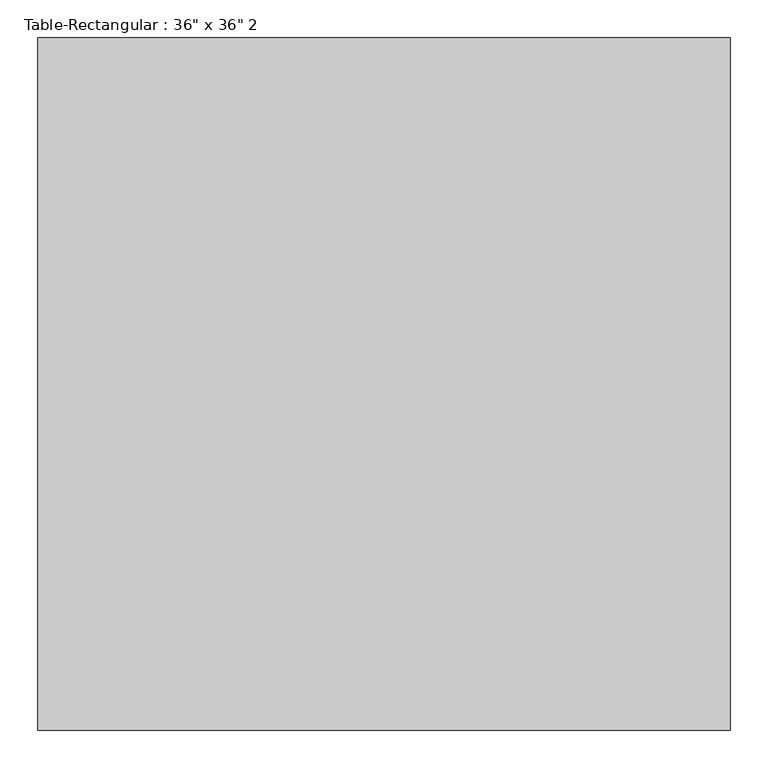
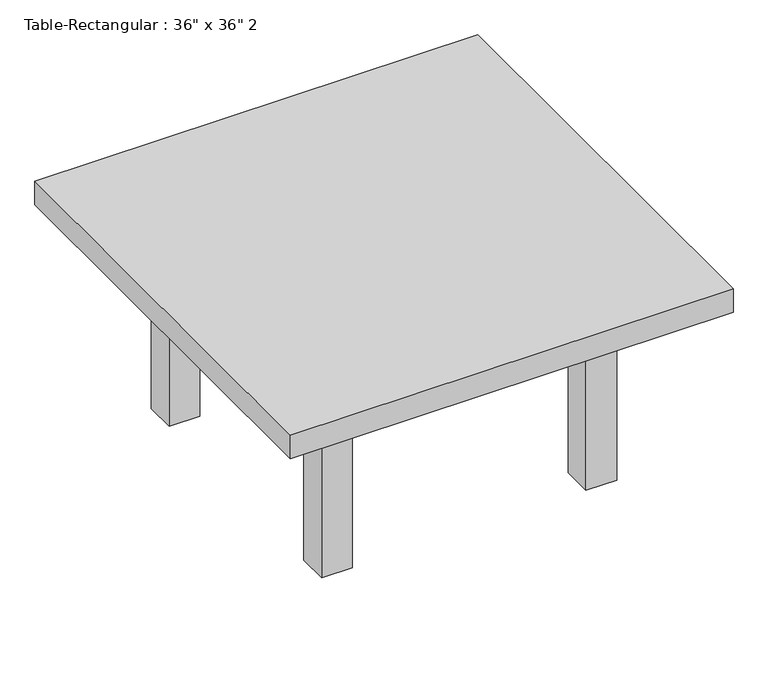
"""IFC4 building model written with IfcOpenShell, lengths in millimetres: furniture geometry."""

from ifc_helpers import new_model, si_unit, frame, origin, origin_with_axes, place, context, project, spatial, polyline, outline, extrude, source, transform, mapped, element, save


def furniture_8a11f05f(model_context):
    return source(origin(), model_context, "Body", "SweptSolid", [
        extrude(outline(polyline([(-241.3, 304.8), (-241.3, 241.3), (-304.8, 241.3), (-304.8, 304.8), (-241.3, 304.8)])), origin_with_axes(), (0.0, 0.0, 1.0), 406.4),
        extrude(outline(polyline([(241.3, 304.8), (304.8, 304.8), (304.8, 241.3), (241.3, 241.3), (241.3, 304.8)])), origin_with_axes(), (0.0, 0.0, 1.0), 406.4),
        extrude(outline(polyline([(-241.3, -304.8), (-304.8, -304.8), (-304.8, -241.3), (-241.3, -241.3), (-241.3, -304.8)])), origin_with_axes(), (0.0, 0.0, 1.0), 406.4),
        extrude(outline(polyline([(241.3, -304.8), (241.3, -241.3), (304.8, -241.3), (304.8, -304.8), (241.3, -304.8)])), origin_with_axes(), (0.0, 0.0, 1.0), 406.4),
        extrude(outline(polyline([(457.2, 457.2), (457.2, -457.2), (-457.2, -457.2), (-457.2, 457.2), (457.2, 457.2)])), frame((0.0, 0.0, 406.4), z_axis=(0.0, 0.0, 1.0), x_axis=(1.0, 0.0, 0.0)), (0.0, 0.0, 1.0), 50.8),
        extrude(outline(polyline([(241.3, 266.7), (241.3, 241.3), (-241.3, 241.3), (-241.3, 266.7), (241.3, 266.7)])), frame((0.0, 0.0, 304.8), z_axis=(0.0, 0.0, 1.0), x_axis=(1.0, 0.0, 0.0)), (0.0, 0.0, 1.0), 101.6),
        extrude(outline(polyline([(241.3, -266.7), (-241.3, -266.7), (-241.3, -241.3), (241.3, -241.3), (241.3, -266.7)])), frame((0.0, 0.0, 304.8), z_axis=(0.0, 0.0, 1.0), x_axis=(1.0, 0.0, 0.0)), (0.0, 0.0, 1.0), 101.6),
        extrude(outline(polyline([(-254.0, -241.3), (-279.4, -241.3), (-279.4, 241.3), (-254.0, 241.3), (-254.0, -241.3)])), frame((0.0, 0.0, 304.8), z_axis=(0.0, 0.0, 1.0), x_axis=(1.0, 0.0, 0.0)), (0.0, 0.0, 1.0), 101.6),
        extrude(outline(polyline([(254.0, -241.3), (254.0, 241.3), (279.4, 241.3), (279.4, -241.3), (254.0, -241.3)])), frame((0.0, 0.0, 304.8), z_axis=(0.0, 0.0, 1.0), x_axis=(1.0, 0.0, 0.0)), (0.0, 0.0, 1.0), 101.6),
    ])


if __name__ == "__main__":
    model = new_model("IFC4")
    model_context = context("Model", 3, world=origin())
    ifc_project = project(units=[si_unit("LENGTHUNIT", "METRE", prefix="MILLI")], contexts=[model_context])
    site = spatial("IfcSite", under=ifc_project)
    building = spatial("IfcBuilding", under=site)
    placement = place(None, origin())
    furniture_shape = furniture_8a11f05f(model_context)
    element("IfcFurniture", 1, ObjectType="Table-Rectangular : 36\" x 36\" 2", at=placement, inside=building, context=model_context, shape_type="MappedRepresentation", body=[
        mapped(furniture_shape, transform((0.0, 0.0, 0.0), x_axis=(1.0, 0.0, 0.0), y_axis=(0.0, 1.0, 0.0), z_axis=(0.0, 0.0, 1.0))),
    ])
    save(model, "model.ifc")

# Revit data of these elements
# Type "Table-Rectangular : 36\" x 36\" 2"
#   Assembly Code = "E2020200"
#   Height = 1' - 6"
#   Length = 3' - 0"
#   Width = 3' - 0"
#   Base Material = Birch
#   Top Material = Birch
#   Default Elevation = 0
# Element 1 (IfcFurniture, "Table-Rectangular : 36\" x 36\" 2")
#   Materials on its faces: "Birch"
# Materials
#   "Birch": class "Wood", colour RGB 224 178 126, transparency 0, Description = "Betula Alleghaniensis", Cost = 0
